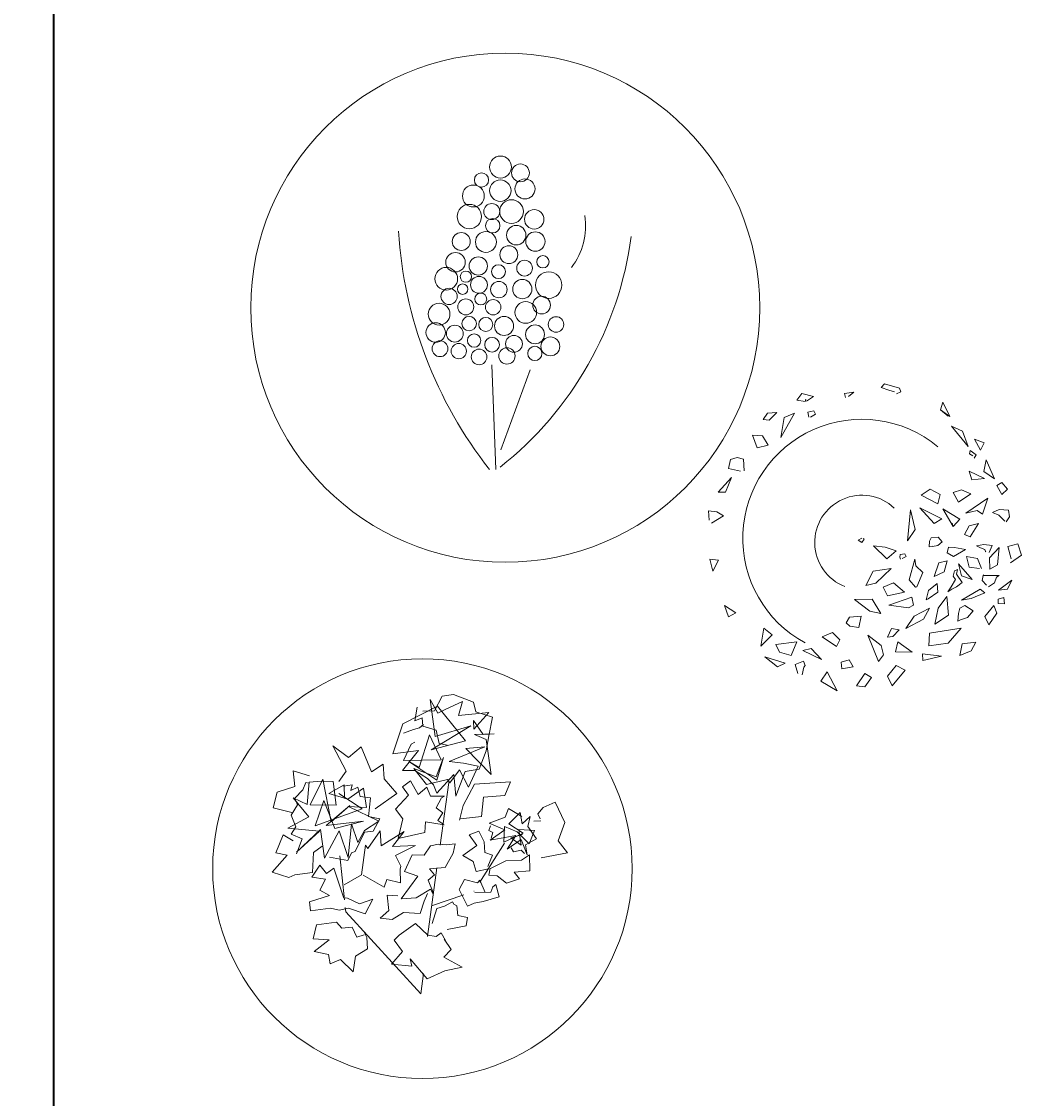
# Model space of a CAD drawing. Units: inches. Extents: x 8049 to 8459, y 820 to 1350.
# Tile 5 of 25: x 8083 to 8109, y 877 to 905. Entities that reach past the tile are written whole.
import ezdxf

# ---------------------------------------------------------------- set-up
doc = ezdxf.new("R2010")
doc.units = ezdxf.units.IN
doc.header["$MEASUREMENT"] = 0
for name, color, linetype, lineweight in [('A-ANNO-DIMS', 2, 'Continuous', 18), ('C-SITE-WALL', 7, 'Continuous', 35), ('zelen', 69, 'Continuous', 13)]:
    doc.layers.add(name, color=color, linetype=linetype, lineweight=lineweight)
doc.styles.get("Standard").update_dxf_attribs({"font": 'arial.ttf'})
doc.dimstyles.get("Standard").update_dxf_attribs({"dimtxt": 0.18, "dimasz": 0.18, "dimexe": 0.18, "dimexo": 0.0625, "dimgap": 0.09, "dimtad": 0, "dimtih": 1, "dimtoh": 1, "dimdec": 4, "dimzin": 0, "dimdsep": 46, "dimtxsty": 'Standard', "dimcen": 0.09, "dimadec": 0, "dimazin": 0, "dimtfac": 1, "dimtdec": 4, "dimtofl": 0, "dimtmove": 0, "dimatfit": 3, "dimfxl": 1, "dimtolj": 1, "dimtzin": 0, "dimarcsym": 0})

# ---------------------------------------------------------------- blocks, each defined once
blk = doc.blocks.new('z_05')
for p, q in [((47.7, 413.4), (29.2, 377.9)), ((74.4, 417.3), (47.7, 413.4)), ((122.3, 398.9), (74.4, 417.3)), ((36.3, 389.4), (-47, 347)), ((-12.6, 387.1), (-18.2, 353.9)), ((18.3, 405.2), (30.8, 316.1)), ((36.6, 372.7), (18.3, 405.2)), ((103.3, 306), (36.3, 389.4)), ((95.8, 400.3), (55.9, 381.9)), ((86.6, 366.4), (95.8, 400.3)), ((127.9, 375.3), (122.3, 398.9)), ((-18.2, 353.9), (-1, 361.5)), ((-1, 361.5), (0.6, 341.4)), ((29.2, 377.9), (0.9, 377.3)), ((55.9, 381.9), (36.6, 372.7)), ((158.8, 374.3), (86.6, 366.4)), ((122.8, 334.2), (158.8, 374.3)), ((168.1, 362.8), (127.9, 375.3)), ((159.1, 318.4), (168.1, 362.8)), ((-47, 347), (-70.6, 274.7)), ((-21.4, 333.2), (-6.8, 337.2)), ((-6.8, 337.2), (2.7, 345.1)), ((0.6, 341.4), (32.6, 331.6)), ((116, 342.1), (21, 284.9)), ((30.8, 316.1), (116, 342.1)), ((122.6, 354.6), (122.8, 334.2)), ((145.3, 321.4), (122.6, 354.6)), ((-45.7, 324.7), (-21.4, 333.2)), ((17, 320.7), (-8.1, 242.2)), ((44.8, 260.6), (17, 320.7)), ((32.6, 331.6), (40.3, 300)), ((124.7, 321.1), (172, 322.7)), ((153, 309.2), (124.7, 321.1)), ((172, 322.7), (145.3, 321.4)), ((152.5, 282), (159.1, 318.4)), ((-214.6, 294.2), (-182.9, 233.1)), ((-176.8, 265.8), (-214.6, 294.2)), ((-147, 291.7), (-176.8, 265.8)), ((-122.2, 232.2), (-147, 291.7)), ((-26.7, 298.1), (-45.4, 258.6)), ((-17.9, 303), (-26.7, 298.1)), ((21, 284.9), (103.3, 306)), ((40.3, 300), (59.6, 295.4)), ((63.8, 256.3), (149.6, 291.5)), ((149.6, 291.5), (103.8, 287.6)), ((103.8, 287.6), (164.9, 225.4)), ((164.9, 225.4), (153, 309.2)), ((-70.6, 274.7), (-9.7, 283.3)), ((-9.7, 283.3), (-47.6, 235.3)), ((-45.4, 258.6), (44.8, 260.6)), ((50.3, 265.9), (32.6, 220.2)), ((34.5, 212), (50.3, 265.9)), ((136.1, 238.6), (152.5, 282)), ((-309.5, 234.4), (-305.8, 197.1)), ((-270.2, 222.5), (-309.5, 234.4)), ((-182.9, 233.1), (-200.1, 208.7)), ((-93.7, 249.9), (-122.2, 232.2)), ((-92, 215.4), (-93.7, 249.9)), ((-47.6, 235.3), (-18.5, 235)), ((-32.2, 256.7), (34.5, 212)), ((-8.1, 242.2), (-32.2, 256.7)), ((-20.6, 240.2), (9.6, 201.8)), ((32.6, 220.2), (-20.6, 240.2)), ((-18.5, 235), (12, 215.9)), ((98.5, 252.7), (63.8, 256.3)), ((65.9, 205.1), (89, 236.9)), ((79.7, 173.9), (102.7, 232.4)), ((89, 236.9), (110.4, 195.2)), ((133.2, 245.8), (98.5, 252.7)), ((102.7, 232.4), (136.1, 238.6)), ((110.4, 195.2), (133.2, 245.8)), ((-286.6, 188.7), (-279, 206.4)), ((-279, 206.4), (-271.8, 204.4)), ((-275.9, 153.5), (-271.1, 207)), ((-271.1, 207), (-242.8, 209.3)), ((-269.3, 152.8), (-238.3, 213.9)), ((-242.8, 209.3), (-214.2, 208.4)), ((-238.3, 213.9), (-219, 112.4)), ((-214.2, 208.4), (-206.8, 152.2)), ((-61.3, 180), (-92, 215.4)), ((-28.6, 209.9), (-48, 196.2)), ((-10, 177.5), (-28.6, 209.9)), ((9.6, 201.8), (59.9, 213.6)), ((12, 215.9), (26.8, 200.5)), ((34.5, 180.8), (74.9, 225.8)), ((59.9, 213.6), (65.9, 205.1)), ((74.9, 225.8), (79.7, 173.9)), ((211.1, 208.1), (125, 202.6)), ((197.5, 175.4), (211.1, 208.1)), ((-348.1, 183.4), (-357.4, 145.5)), ((-305.8, 197.1), (-348.1, 183.4)), ((-305.7, 168.7), (-286.6, 188.7)), ((-187.8, 200.8), (-224.5, 180.1)), ((-188.9, 197.7), (-168.6, 200.5)), ((-187, 168.3), (-187.8, 200.8)), ((-178.5, 166), (-140.9, 192.9)), ((-168.6, 200.5), (-171.2, 187.4)), ((-171.2, 187.4), (-155.1, 195.5)), ((-155.1, 195.5), (-149.1, 172.6)), ((-140.9, 192.9), (-133.8, 146.3)), ((-48, 196.2), (-33.6, 175.7)), ((10.9, 194.8), (-10, 177.5)), ((19.4, 173.3), (10.9, 194.8)), ((26.8, 200.5), (34.5, 180.8)), ((42.3, 56.3), (63, 206.2)), ((125, 202.6), (98, 151)), ((-309.5, 169.9), (-275.9, 153.5)), ((-272.4, 123.9), (-309.5, 169.9)), ((-299.4, 152.8), (-305.7, 168.7)), ((-236.2, 163), (-257.1, 102.9)), ((-210, 96), (-236.2, 163)), ((-224.5, 180.1), (-178.5, 166)), ((-144.4, 143), (-200.5, 180.1)), ((-149.1, 172.6), (-124.4, 169.6)), ((-124.4, 169.6), (-129.3, 125.2)), ((-113.4, 143.1), (-61.3, 180)), ((-33.6, 175.7), (-64.3, 142.3)), ((53.3, 173.7), (19.4, 173.3)), ((33.2, 145.5), (45.7, 169.6)), ((45.7, 169.6), (53.3, 173.7)), ((141.3, 124.8), (146.2, 170.9)), ((146.2, 170.9), (197.5, 175.4)), ((318.2, 159), (289, 146.8)), ((341.6, 110.1), (318.2, 159)), ((-357.4, 145.5), (-313.2, 134.2)), ((-314.6, 127.8), (-299.4, 152.8)), ((-206.8, 152.2), (-269.3, 152.8)), ((-257.1, 102.9), (-144.4, 143)), ((-174.3, 151.5), (-230.4, 103.2)), ((-219, 112.4), (-174.3, 151.5)), ((-177.2, 148.6), (-104.7, 113.7)), ((-133.8, 146.3), (-177.2, 148.6)), ((-64.3, 142.3), (-46.8, 118.9)), ((49.2, 133.6), (33.2, 145.5)), ((36.7, 115.6), (49.2, 133.6)), ((98, 151), (88.7, 115.9)), ((198.5, 123.6), (206.2, 144.3)), ((206.2, 144.3), (238.2, 125.2)), ((207.2, 107.5), (234.5, 134.4)), ((234.5, 134.4), (238.7, 107.5)), ((289, 146.8), (276.7, 130.9)), ((276.7, 130.9), (282.3, 119)), ((-322.2, 96.6), (-272.4, 123.9)), ((-303.6, 100.1), (-314.6, 127.8)), ((-230.4, 103.2), (-141.2, 113.4)), ((-141.2, 113.4), (-210, 96)), ((-170.3, 107.2), (-177.7, 26.3)), ((-154.7, 62.5), (-170.3, 107.2)), ((-104.7, 113.7), (-138.8, 91.1)), ((-129.3, 125.2), (-102.3, 118.9)), ((-102.3, 118.9), (-117.9, 89.5)), ((-46.8, 118.9), (-58.1, 72.1)), ((5.6, 86.3), (7.6, 111.7)), ((7.6, 111.7), (51.8, 105.2)), ((48.6, 107.6), (36.7, 115.6)), ((91.6, 119.6), (141.3, 124.8)), ((159.9, 108.8), (198.5, 123.6)), ((197.7, 92.7), (159.9, 108.8)), ((241.1, 84.8), (207.2, 107.5)), ((238.7, 107.5), (258, 124.6)), ((258, 124.6), (252.2, 100.6)), ((284.1, 114.7), (267.1, 113.5)), ((324.9, 66.8), (341.6, 110.1)), ((-333.3, 80.8), (-351, 37.5)), ((-309.7, 66.5), (-333.3, 80.8)), ((-247, 90.1), (-322.2, 96.6)), ((-314.4, 82.9), (-303.6, 100.1)), ((-288, 71.4), (-314.4, 82.9)), ((-244.4, 93.4), (-301.8, 39.5)), ((-301.8, 39.5), (-247, 90.1)), ((-234.9, 25.3), (-244.4, 93.4)), ((-199.4, 90.7), (-234.9, 25.3)), ((-177.7, 26.3), (-199.4, 90.7)), ((-138.6, 87.7), (-161.1, 41.4)), ((-138.8, 91.1), (-154.7, 62.5)), ((-117.9, 89.5), (-138.6, 87.7)), ((-130.7, 48.4), (-100.9, 90.4)), ((-100.9, 90.4), (-98.5, 54.7)), ((-98.5, 54.7), (-43.7, 88.9)), ((-43.7, 88.9), (-71.8, 53.1)), ((-58.1, 72.1), (5.6, 86.3)), ((135.5, 89.5), (111.9, 81.1)), ((111.9, 81.1), (130.2, 55.1)), ((148.3, 64.3), (135.5, 89.5)), ((163.2, 102.8), (159.3, 91.6)), ((159.3, 91.6), (169, 86.6)), ((162.5, 68.1), (197.7, 92.7)), ((223.6, 79.6), (162.5, 68.1)), ((169, 86.6), (165, 72.9)), ((196.9, 101.2), (195.1, 63.5)), ((195.1, 63.5), (241.1, 84.8)), ((226.8, 87.8), (196.9, 101.2)), ((203.3, 46.4), (223.6, 79.6)), ((239.5, 81.5), (211.5, 73.6)), ((255.9, 59.2), (226.8, 87.8)), ((231.3, 94), (268.9, 91.4)), ((236.9, 55.9), (231.3, 94)), ((252.2, 100.6), (273.6, 71.3)), ((268.9, 91.4), (255.9, 59.2)), ((-302, 35.3), (-288, 71.4)), ((-260.8, 38.4), (-240.2, 53.7)), ((-145.9, -14.9), (-136.6, 56.2)), ((-136.6, 56.2), (-130.7, 48.4)), ((-71.8, 53.1), (-16.6, 55.1)), ((-16.6, 55.1), (-64.6, 31.5)), ((19, 54.4), (4.5, 32.1)), ((38.8, 58.6), (19, 54.4)), ((57.8, 57), (38.8, 58.6)), ((78.7, 59.7), (57.8, 57)), ((73.6, 37.4), (78.7, 59.7)), ((130.2, 55.1), (97.1, 31.2)), ((137.3, -32.7), (196.8, 60.8)), ((149.9, 38.3), (148.3, 64.3)), ((236.3, 69.4), (203.3, 46.4)), ((211.5, 73.6), (236.9, 55.9)), ((250.9, 32.9), (236.3, 69.4)), ((273.6, 71.3), (246.7, 57.2)), ((246.7, 57.2), (250.9, 32.9)), ((347.5, 37.8), (324.9, 66.8)), ((-324.2, 32.6), (-360.1, -8.6)), ((-351, 37.5), (-324.2, 32.6)), ((-263.3, -9.2), (-260.8, 38.4)), ((-179.1, 19.6), (-222.6, 27.6)), ((-197.6, 30.4), (-186.7, -75.1)), ((-170.2, 37.7), (-179.1, 19.6)), ((-161.1, 41.4), (-170.2, 37.7)), ((-64.6, 31.5), (-51.4, 5.7)), ((-24.4, 33.3), (-43.1, -6.5)), ((4.5, 32.1), (-24.4, 33.3)), ((54.6, 2.8), (73.6, 37.4)), ((97.1, 31.2), (121.2, 16.7)), ((168.1, 32.5), (149.9, 38.3)), ((156.5, 4.8), (168.1, 32.5)), ((218.6, 40.3), (212.6, 49.9)), ((236.5, 44), (218.6, 40.3)), ((244.2, 36.6), (236.5, 44)), ((237.6, 20.3), (256.2, 32.8)), ((256.2, 32.8), (257.4, -5.3)), ((284.6, 26.2), (347.5, 37.8)), ((-246.1, 8.6), (-264.6, -20.3)), ((-229.7, -11.4), (-246.1, 8.6)), ((-212.5, 1.1), (-229.7, -11.4)), ((-188.1, -70.9), (-212.5, 1.1)), ((-51.4, 5.7), (-53.3, -1)), ((12.2, -162.5), (34.8, 2)), ((17.3, -0.7), (54.6, 2.8)), ((121.2, 16.7), (128.5, -6.7)), ((159.5, -16), (162.4, 0.9)), ((163.5, 0), (199.5, 18.3)), ((199.5, 18.3), (237.6, 20.3)), ((-360.1, -8.6), (-319.8, -21.4)), ((-319.8, -21.4), (-305.8, -15)), ((-305.8, -15), (-263.3, -9.2)), ((-264.6, -20.3), (-232.2, -25.5)), ((-232.2, -25.5), (-245.8, -51.9)), ((-187.7, -38.6), (-145.9, -14.9)), ((-91.7, -44.5), (-142, -16)), ((-53.3, -1), (-52.3, -34)), ((-11.2, -18.3), (-50.9, -72.3)), ((-43.1, -6.5), (-11.2, -18.3)), ((14.1, -27.4), (28.8, -14.9)), ((28.8, -14.9), (17.3, -0.7)), ((128.5, -6.7), (158.7, -0.6)), ((179.2, -17.2), (159.5, -16)), ((201.2, -35.1), (179.2, -17.2)), ((232.4, -24.4), (201.2, -35.1)), ((257.4, -5.3), (219.7, -8.5)), ((219.7, -8.5), (232.4, -24.4)), ((-85.5, -25.9), (-91.7, -44.5)), ((-52.3, -34), (-85.5, -25.9)), ((-15.2, -70.2), (19.4, -49.1)), ((25.9, -56.8), (14.1, -27.4)), ((19.4, -49.1), (24.6, -59.5)), ((88.3, -50.2), (101.1, -26.2)), ((107.8, -89.9), (88.3, -50.2)), ((101.1, -26.2), (131.6, -34.3)), ((131.6, -34.3), (137.9, -27.4)), ((137.9, -27.4), (150.4, -57.2)), ((163.6, -56.6), (168.4, -43.5)), ((168.4, -43.5), (176.2, -37.8)), ((176.2, -37.8), (183.5, -67.3)), ((-222.9, -64.1), (-270.2, -79.3)), ((-245.8, -51.9), (-222.9, -64.1)), ((-179.4, -70.6), (-185, -70.2)), ((-151.1, -84.7), (-179.4, -70.6)), ((-119.1, -72.9), (-151.1, -84.7)), ((-137, -108.6), (-119.1, -72.9)), ((-84.6, -63.8), (-80.4, -99.9)), ((-59, -65.1), (-84.6, -63.8)), ((-50.9, -72.3), (-15.2, -70.2)), ((3.9, -77.8), (12.1, -59.8)), ((99.1, -62.5), (22.1, -89.1)), ((123.4, -54.1), (123.7, -54)), ((125.8, -57.1), (163.6, -56.6)), ((183.5, -67.3), (145.4, -78.6)), ((-270.2, -79.3), (-268.3, -101.3)), ((-268.3, -101.3), (-219.9, -94.9)), ((-219.9, -94.9), (-199.8, -99.2)), ((-199.8, -99.2), (-177.4, -94.6)), ((-184.9, -93), (-183.8, -103.6)), ((-177.4, -94.6), (-137, -108.6)), ((-80.4, -99.9), (-101.4, -118.3)), ((-5.1, -107.6), (3.9, -77.8)), ((34.7, -95.4), (23.5, -131.1)), ((52.8, -90), (34.7, -95.4)), ((72.1, -79.9), (52.8, -90)), ((75, -85.4), (72.1, -79.9)), ((82.5, -89.1), (75, -85.4)), ((85.1, -112.3), (82.5, -89.1)), ((124.2, -82.4), (107.8, -89.9)), ((145.4, -78.6), (124.2, -82.4)), ((-205.8, -128), (-253.7, -134.6)), ((-192.7, -142.7), (-205.8, -128)), ((-183.8, -103.6), (-3.6, -299.6)), ((-101.4, -118.3), (-72.6, -121.5)), ((-72.6, -121.5), (-45.6, -105.4)), ((-45.6, -105.4), (-5.1, -107.6)), ((108, -117.3), (85.1, -112.3)), ((104.9, -137.2), (108, -117.3)), ((-253.7, -134.6), (-261.4, -168.3)), ((-168.7, -140.1), (-192.7, -142.7)), ((-157, -164.4), (-168.7, -140.1)), ((-133.5, -165.3), (-138.4, -154.1)), ((-16.2, -131.7), (-55.5, -159.5)), ((13.1, -159.3), (-16.2, -131.7)), ((45, -154.1), (32.6, -162.8)), ((55.2, -172.3), (45, -154.1)), ((59.4, -145.7), (104.9, -137.2)), ((-261.4, -168.3), (-223.5, -170.8)), ((-223.5, -170.8), (-259.2, -198.1)), ((-139.9, -158.9), (-157, -164.4)), ((-131.8, -192.3), (-133.5, -165.3)), ((-55.5, -159.5), (-67.8, -171.1)), ((-67.8, -171.1), (-47.6, -198.1)), ((32.6, -162.8), (13.1, -159.3)), ((69.1, -193.4), (52.3, -169.2)), ((-259.2, -198.1), (-224.7, -206)), ((-224.7, -206), (-221.4, -228.1)), ((-160.4, -209.4), (-131.8, -192.3)), ((-47.6, -198.1), (-74.3, -229.2)), ((51.3, -211.7), (69.1, -193.4)), ((-221.4, -228.1), (-196.4, -217.5)), ((-196.4, -217.5), (-166.3, -247.2)), ((-166.3, -247.2), (-160.4, -209.4)), ((-74.3, -229.2), (-25.6, -233.9)), ((-29.7, -216.4), (11.5, -264)), ((-25.6, -233.9), (-29.7, -216.4)), ((95.2, -236.2), (51.3, -211.7)), ((2.5, -250.9), (-3.6, -299.6)), ((11.5, -264), (54, -244.9)), ((54, -244.9), (95.2, -236.2))]:
    blk.add_line(p, q)
blk.add_circle((0, 0), 502.5)
blk = doc.blocks.new('z_06')
for p, q in [((-26, -111.8), (-18.2, -317.4)), ((48.7, -121.5), (-8.6, -278.6))]:
    blk.add_line(p, q)
for centre, radius in [((0, 0), 499.1), ((-9.3, 275.8), 21.5), ((29.8, 264.3), 17.5), ((-46.5, 250.4), 14), ((-62.5, 219), 21.4), ((-9.7, 229.6), 21.1), ((38.7, 232.9), 19.7), ((12.3, 188.5), 23.2), ((-70.3, 178.8), 23.9), ((-26.4, 188.5), 15.7), ((56.9, 173.3), 19), ((-24.6, 160.8), 14.2), ((-37.9, 128.9), 20.5), ((21.6, 142.3), 19.1), ((59.1, 129.8), 19), ((-86.3, 129.8), 17.6), ((-97.5, 89.2), 19.1), ((7.1, 104), 17.6), ((-52.8, 81.8), 18), ((37.9, 77.6), 15.4), ((74, 90.1), 12), ((-115.7, 56.8), 22.2), ((-77, 60.9), 11.1), ((-13.1, 70.7), 13.7), ((85.2, 44.4), 26), ((-83.5, 36.4), 10.2), ((-51.5, 44.9), 16.6), ((-12.5, 35.6), 16.1), ((33.5, 36.5), 18.9), ((-110.1, 22.2), 15.9), ((-47.9, 17.1), 11.7), ((71.4, 5.1), 17.3), ((-129.8, -12.5), 21.4), ((-77.3, 1.7), 15.7), ((-23.7, 1), 15.1), ((40.2, -9.2), 21.3), ((-70.8, -31.2), 14.2), ((-38.2, -32.7), 13.7), ((-2.3, -35.8), 18.7), ((99.7, -32.8), 15.2), ((-136.5, -48.5), 19.1), ((-98.8, -50.8), 16.5), ((58.4, -52.2), 18.5), ((-61.1, -64.4), 13.1), ((-25.8, -72.6), 14.4), ((17.1, -70.7), 16.5), ((88.5, -75.8), 18.5), ((-128, -80.4), 15.5), ((-91.1, -85.1), 15), ((-51.3, -96.5), 15.3), ((3.4, -94.5), 16), ((58, -89.6), 14)]:
    blk.add_circle(centre, radius)
for centre, radius, start, end in [((21.1, 161.1), 136.5, 323.03, 8.2301), ((631.6, 203.5), 842.7, 183.6263, 218.177), ((-440.2, 231.1), 693.3, 308.3911, 352.4108)]:
    blk.add_arc(centre, radius, start, end)
blk = doc.blocks.new('z_66')
for p, q in [((83.2, 488.9), (72.7, 477.7)), ((72.7, 477.7), (96.4, 469.7)), ((129.8, 476.2), (83.2, 488.9)), ((134, 464.6), (129.8, 476.2)), ((-176.4, 458.5), (-191.7, 438.6)), ((-191.7, 438.6), (-165.6, 433.5)), ((-139.2, 449.4), (-176.4, 458.5)), ((-165.6, 433.5), (-163.6, 441.1)), ((-161.1, 434.6), (-139.2, 449.4)), ((-13.6, 463.6), (-42.5, 459.2)), ((-42.5, 459.2), (-39.3, 446.9)), ((-30.3, 449.4), (-13.6, 463.6)), ((96.4, 469.7), (114.5, 463.9)), ((114.5, 463.9), (114.5, 463.9)), ((120.4, 457.8), (134, 464.6)), ((-165.6, 433.5), (-165.6, 433.5)), ((-138.9, 404.9), (-156.9, 400.2)), ((-133.3, 394.8), (-138.9, 404.9)), ((265.2, 432.1), (258.2, 407.5)), ((258.2, 407.5), (287.4, 387.2)), ((258.2, 407.5), (281.9, 388.6)), ((287.4, 387.2), (265.2, 432.1)), ((-283.6, 397.7), (-297.2, 378.2)), ((-297.2, 378.2), (-277.7, 376)), ((-254, 399.9), (-283.6, 397.7)), ((-277.7, 376), (-272.8, 380.7)), ((-272.8, 380.7), (-254, 399.9)), ((-241.9, 321.7), (-199.1, 397.3)), ((-231.4, 383.6), (-241.9, 321.7)), ((-199.1, 397.3), (-231.4, 383.6)), ((-156.9, 400.2), (-153.8, 385.4)), ((-148.6, 384.7), (-133.3, 394.8)), ((281.9, 388.6), (281.9, 388.6)), ((344.2, 293.1), (292, 357.2)), ((292, 357.2), (326.8, 341.2)), ((326.8, 341.2), (344.2, 293.1)), ((-330.3, 328.9), (-298.6, 327.1)), ((-316, 288.8), (-330.3, 328.9)), ((-298.6, 327.1), (-280.8, 297.1)), ((383.1, 281.9), (364.4, 316.3)), ((364.4, 316.3), (394.6, 305.1)), ((394.6, 305.1), (383.1, 281.9)), ((-280.8, 297.1), (-316, 288.8)), ((350.8, 280.8), (348.7, 270.3)), ((348.7, 270.3), (358.8, 264.5)), ((369.2, 266.7), (350.8, 280.8)), ((-399.2, 252.6), (-405.8, 224)), ((-377.9, 259.1), (-399.2, 252.6)), ((-358.4, 254), (-377.9, 259.1)), ((-356, 217.5), (-358.4, 254)), ((358.8, 264.5), (358.8, 264.5)), ((363.3, 256.6), (369.2, 266.7)), ((400.9, 251.9), (393.9, 214.6)), ((426.6, 192.2), (400.9, 251.9)), ((-405.8, 224), (-368.2, 216.4)), ((-368.2, 216.4), (-368.2, 216.4)), ((348, 215.7), (356, 188.9)), ((395.3, 193.2), (348, 215.7)), ((393.9, 214.6), (426.6, 192.2)), ((-396.4, 196.1), (-438.1, 150.2)), ((-414.8, 150.9), (-396.4, 196.1)), ((356, 188.9), (395.3, 193.2)), ((450, 180.6), (434.3, 171.2)), ((434.3, 171.2), (449.6, 142.6)), ((467.7, 160.3), (450, 180.6)), ((-438.1, 150.2), (-414.8, 150.9)), ((225.2, 159.9), (197, 140.8)), ((197, 140.8), (249.5, 113.6)), ((256.8, 142.6), (225.2, 159.9)), ((249.5, 113.6), (256.8, 142.6)), ((323.6, 157.8), (297.5, 149.8)), ((297.5, 149.8), (314.6, 119.4)), ((314.6, 119.4), (352.9, 145.5)), ((352.9, 145.5), (323.6, 157.8)), ((449.6, 142.6), (467.7, 160.3)), ((193.1, 101.3), (238, 52.1)), ((261.7, 66.6), (193.1, 101.3)), ((336.9, 84.3), (405.8, 131.7)), ((405.8, 131.7), (389.8, 82.1)), ((-468.4, 91.6), (-466.3, 62.6)), ((-441.6, 89), (-468.4, 91.6)), ((-458.3, 53.9), (-421.1, 76)), ((-421.1, 76), (-441.6, 89)), ((164.3, 94.8), (154.2, -2.2)), ((178.9, 33.3), (164.3, 94.8)), ((265.2, 98.8), (297.2, 42.7)), ((318.8, 66.2), (265.2, 98.8)), ((372.7, 93), (336.9, 84.3)), ((389.8, 82.1), (372.7, 93)), ((441.6, 95.9), (420.7, 86.5)), ((420.7, 86.5), (440.2, 78.5)), ((440.2, 78.5), (459.7, 59.7)), ((470.5, 93.7), (441.6, 95.9)), ((463.2, 57.9), (474, 73.5)), ((474, 73.5), (470.5, 93.7)), ((-466.3, 62.6), (-466.3, 62.6)), ((238, 52.1), (261.7, 66.6)), ((297.2, 42.7), (294.1, 53.6)), ((297.2, 42.7), (318.8, 66.2)), ((347.3, 45.2), (332.7, 18.1)), ((376.9, 52.5), (347.3, 45.2)), ((350.8, 10.9), (376.9, 52.5)), ((459.7, 59.7), (459.7, 59.7)), ((11.8, 6.2), (0, 0)), ((0, 0), (12.2, -6.9)), ((12.2, -6.9), (19.1, 2.9)), ((19.1, 2.9), (15.7, 5.8)), ((154.2, -2.2), (178.9, 33.3)), ((229, 7.2), (223.1, -2.5)), ((250.6, 9.8), (229, 7.2)), ((263.4, -5.4), (250.6, 9.8)), ((332.7, 18.1), (350.8, 10.9)), ((84.6, -21.7), (48, -17)), ((48, -17), (90.1, -58.3)), ((119.4, -32.9), (84.6, -21.7)), ((90.1, -58.3), (119.4, -32.9)), ((223.1, -2.5), (222.7, -20.6)), ((222.7, -20.6), (234.2, -18.1)), ((233.2, -19.9), (249.9, -15.9)), ((234.2, -18.1), (234.2, -18.1)), ((249.9, -15.9), (263.4, -5.4)), ((282.9, -21.3), (279.1, -39.1)), ((302.1, -22.8), (282.9, -21.3)), ((298.6, -50.3), (335.8, -28.6)), ((335.8, -28.6), (302.1, -22.8)), ((393.6, -13), (371, -17)), ((371, -17), (383.5, -23.5)), ((383.5, -23.5), (396.7, -28.9)), ((420, -15.9), (393.6, -13)), ((396.7, -28.9), (398.5, -35.5)), ((410.3, -38), (420, -15.9)), ((442, -22.4), (411.3, -55.4)), ((436, -77.1), (442, -22.4)), ((499.7, -10.9), (468.8, -19.9)), ((468.8, -19.9), (478.8, -58.6)), ((510.9, -47), (499.7, -10.9)), ((-464.2, -59.3), (-436.4, -62.6)), ((-454.5, -96.3), (-464.2, -59.3)), ((-436.4, -62.6), (-454.5, -96.3)), ((131.9, -44.9), (130.2, -52.5)), ((130.2, -52.5), (132.9, -59.3)), ((146.5, -42.3), (131.9, -44.9)), ((138.2, -56.8), (151, -51)), ((151, -51), (146.5, -42.3)), ((177.8, -59), (160.1, -123.8)), ((181, -80.3), (177.8, -59)), ((278.4, -64), (252.6, -70.9)), ((269.7, -98.4), (278.4, -64)), ((279.1, -39.1), (298.6, -50.3)), ((339, -51), (347.7, -84.3)), ((374.1, -56.8), (339, -51)), ((386.3, -87.9), (374.1, -56.8)), ((398.5, -35.5), (399.5, -35.8)), ((411.3, -55.4), (412.7, -90.8)), ((477.5, -70.2), (510.9, -47)), ((478.8, -58.6), (478.8, -58.6)), ((47.7, -96.6), (24, -141.9)), ((104.1, -87.9), (47.7, -96.6)), ((56, -133.9), (104.1, -87.9)), ((202.2, -100.6), (181, -80.3)), ((183.7, -145.5), (202.2, -100.6)), ((252.6, -70.9), (237.7, -112.9)), ((237.7, -112.9), (269.7, -98.4)), ((301.7, -95.5), (297.9, -112.2)), ((310.8, -91.9), (301.7, -95.5)), ((307.6, -106), (310.8, -91.9)), ((314.2, -74.2), (356.7, -123)), ((323.3, -111.1), (314.2, -74.2)), ((347.7, -84.3), (379.7, -88.3)), ((379.7, -88.3), (379.7, -88.3)), ((412.7, -90.8), (436, -77.1)), ((24, -141.9), (56, -133.9)), ((111.4, -132.8), (78.3, -146.2)), ((145.1, -162.1), (111.4, -132.8)), ((160.1, -123.8), (179.6, -146.6)), ((304.5, -123), (291.6, -145.8)), ((297.9, -112.2), (304.5, -123)), ((325.4, -132.4), (307.6, -106)), ((308.3, -145.8), (325.4, -132.4)), ((356.7, -123), (323.3, -111.1)), ((356.7, -123), (356.7, -123)), ((356.7, -123), (356.7, -123)), ((391.2, -110), (388.4, -125.6)), ((388.4, -125.6), (402.3, -140.8)), ((391.2, -110), (393.2, -108.6)), ((441.3, -110), (391.2, -110)), ((407.9, -145.5), (427, -133.5)), ((427, -133.5), (432.9, -115.8)), ((432.9, -115.8), (441.3, -110)), ((480.9, -124.5), (439.2, -156)), ((467.7, -153.4), (480.9, -124.5)), ((78.3, -146.2), (92.2, -174.1)), ((92.2, -174.1), (145.1, -162.1)), ((179.6, -146.6), (183.7, -145.5)), ((220.6, -157), (212.6, -186)), ((219.2, -183.5), (249.2, -162.1)), ((247.1, -135.7), (220.6, -157)), ((249.2, -162.1), (247.1, -135.7)), ((291.6, -145.8), (281.2, -161.8)), ((281.2, -161.8), (293, -152.7)), ((293, -152.7), (308.3, -145.8)), ((382.5, -152.7), (323.3, -187.4)), ((353.9, -182), (396.7, -164.3)), ((396.7, -164.3), (382.5, -152.7)), ((402.3, -140.8), (402.3, -140.8)), ((439.2, -156), (467.7, -153.4)), ((44.5, -184.2), (-10.8, -184.9)), ((-10.8, -184.9), (36.9, -222.2)), ((71, -229.1), (44.5, -184.2)), ((168.1, -178.4), (96.7, -202.6)), ((173, -203.4), (168.1, -178.4)), ((212.6, -186), (219.2, -183.5)), ((277.4, -176.2), (250.2, -212.4)), ((283.3, -233.8), (277.4, -176.2)), ((323.3, -187.4), (353.9, -182)), ((438.5, -183.8), (456.2, -179.1)), ((438.5, -197.6), (438.5, -183.8)), ((458.7, -199), (438.5, -197.6)), ((456.2, -179.1), (458.7, -199)), ((-417.9, -204.1), (-405.1, -239.6)), ((-382.8, -226.5), (-417.9, -204.1)), ((-405.1, -239.6), (-382.8, -226.5)), ((36.9, -222.2), (71, -229.1)), ((96.7, -202.6), (157.6, -211.3)), ((157.6, -211.3), (173, -203.4)), ((223.8, -212.4), (175.4, -237.7)), ((204.3, -246.8), (223.8, -212.4)), ((250.2, -212.4), (240.1, -262.4)), ((240.1, -262.4), (283.3, -233.8)), ((314.6, -228.7), (311.8, -252.6)), ((318.4, -212.1), (314.6, -228.7)), ((334.1, -203.7), (318.4, -212.1)), ((360.2, -221.1), (334.1, -203.7)), ((342.8, -241.4), (360.2, -221.1)), ((425.3, -204.5), (396.7, -238.5)), ((409.2, -264.2), (434.3, -228)), ((434.3, -228), (425.3, -204.5)), ((-26.4, -240.3), (-37.6, -258.4)), ((-37.6, -258.4), (-25.8, -268.5)), ((10.1, -237.7), (-26.4, -240.3)), ((-25.8, -268.5), (2.4, -273.2)), ((-25.8, -268.5), (-25.8, -268.5)), ((-25.8, -268.5), (-25.8, -268.5)), ((2.4, -273.2), (10.1, -237.7)), ((175.4, -237.7), (149.6, -276.1)), ((149.6, -276.1), (204.3, -246.8)), ((311.8, -252.6), (320.5, -249.3)), ((320.5, -249.3), (342.8, -241.4)), ((396.7, -238.5), (409.2, -264.2)), ((-295.1, -275), (-304.2, -331.5)), ((-304.2, -331.5), (-269, -296)), ((-269, -296), (-295.1, -275)), ((-80, -288), (-112.4, -302.5)), ((-112.4, -302.5), (-67.5, -331.8)), ((-56.7, -311.6), (-80, -288)), ((30.6, -297.1), (72.7, -329.3)), ((64, -379.6), (30.6, -297.1)), ((105.1, -276.1), (91.9, -303.6)), ((91.9, -303.6), (108.6, -301.4)), ((128.8, -280.4), (105.1, -276.1)), ((108.6, -301.4), (128.8, -280.4)), ((223.8, -290.2), (221.3, -330)), ((322.2, -275), (223.8, -290.2)), ((282.2, -321.7), (322.2, -275)), ((-191.1, -317.4), (-256.8, -326.4)), ((-256.8, -326.4), (-245.7, -350.3)), ((-209.8, -360.4), (-191.1, -317.4)), ((-67.5, -331.8), (-56.7, -311.6)), ((72.7, -329.3), (79.3, -357.9)), ((117.3, -348.8), (124.2, -317.7)), ((124.2, -317.7), (168.8, -349.9)), ((221.3, -330), (282.2, -321.7)), ((325.7, -323.9), (318.4, -360.1)), ((368.9, -319.2), (325.7, -323.9)), ((354.3, -346.3), (368.9, -319.2)), ((-292, -364.4), (-252, -395.5)), ((-228.3, -383.9), (-292, -364.4)), ((-245.7, -350.3), (-209.8, -360.4)), ((-172.6, -344.9), (-146.9, -338.7)), ((-114.8, -372.7), (-172.6, -344.9)), ((-146.9, -338.7), (-114.8, -372.7)), ((79.3, -357.9), (64, -379.6)), ((168.8, -349.9), (117.3, -348.8)), ((201.8, -355), (202.2, -376.3)), ((261, -362.2), (201.8, -355)), ((202.2, -376.3), (261, -362.2)), ((318.4, -360.1), (354.3, -346.3)), ((-252, -395.5), (-228.3, -383.9)), ((-197.3, -388.3), (-171.2, -377.8)), ((-188.3, -416.9), (-197.3, -388.3)), ((-169.5, -396.6), (-174.7, -420.5)), ((-171.2, -377.8), (-166, -391.5)), ((-166, -391.5), (-169.5, -396.6)), ((-27.8, -374.5), (-52.9, -381.8)), ((-52.9, -381.8), (-50.8, -402)), ((-50.8, -402), (-15.3, -396.2)), ((-15.3, -396.2), (-27.8, -374.5)), ((91.9, -424.8), (119, -391.5)), ((119, -391.5), (146.9, -406.4)), ((-174.7, -420.5), (-174.7, -420.5)), ((-116.2, -441.1), (-96.4, -411.8)), ((-96.4, -411.8), (-65.8, -470.8)), ((21.6, -417.2), (-4.5, -455.6)), ((42.1, -428.8), (21.6, -417.2)), ((21.6, -458.1), (42.1, -428.8)), ((106.8, -455.6), (91.9, -424.8)), ((146.9, -406.4), (106.8, -455.6)), ((-65.8, -470.8), (-116.2, -441.1)), ((-4.5, -455.6), (21.6, -458.1))]:
    blk.add_line(p, q)
for centre, radius, start, end in [((11.8, 6.2), 372.3, 50.2118, 241.5185), ((12.2, -6.9), 147.8, 46.7611, 248.9067)]:
    blk.add_arc(centre, radius, start, end)
blk = doc.blocks.new('*D50')
at = {"layer": 'A-ANNO-DIMS', "color": 0, "lineweight": -2, "transparency": 16777216}
for p, q in [((8083.335, 1045.871), (8049.617, 1045.871)), ((8049.797, 1045.691), (8049.797, 945.553)), ((8049.797, 845.051), (8049.797, 945.189)), ((8074.335, 844.871), (8049.617, 844.871))]:
    blk.add_line(p, q, dxfattribs=at)
at = {"layer": 'A-ANNO-DIMS', "color": 0, "transparency": 16777216}
for points in [[(8049.767, 1045.691), (8049.827, 1045.691), (8049.797, 1045.871)], [(8049.767, 845.051), (8049.827, 845.051), (8049.797, 844.871)]]:
    blk.add_solid(points, dxfattribs=at)
at = {"layer": 'Defpoints', "color": 0, "transparency": 16777216}
for p in [(8049.797, 1045.871), (8083.397, 1045.871), (8074.397, 844.871)]:
    blk.add_point(p, dxfattribs=at)
at = {"layer": 'A-ANNO-DIMS', "color": 0, "transparency": 16777216, "insert": (8049.797, 945.371), "char_height": 0.18, "attachment_point": 5}
blk.add_mtext('\\A1;201', dxfattribs=at)
blk = doc.blocks.new('*D70')
at = {"layer": 'A-ANNO-DIMS', "color": 0, "lineweight": -2, "transparency": 16777216}
for p, q in [((8083.397, 1045.808), (8083.397, 820.091)), ((8137.397, 1045.808), (8137.397, 820.091)), ((8083.577, 820.271), (8110.179, 820.271)), ((8137.217, 820.271), (8110.616, 820.271))]:
    blk.add_line(p, q, dxfattribs=at)
at = {"layer": 'A-ANNO-DIMS', "color": 0, "transparency": 16777216}
for points in [[(8083.577, 820.301), (8083.577, 820.241), (8083.397, 820.271)], [(8137.217, 820.301), (8137.217, 820.241), (8137.397, 820.271)]]:
    blk.add_solid(points, dxfattribs=at)
at = {"layer": 'Defpoints', "color": 0, "transparency": 16777216}
for p in [(8083.397, 1045.871), (8137.397, 1045.871), (8083.397, 820.271)]:
    blk.add_point(p, dxfattribs=at)
at = {"layer": 'A-ANNO-DIMS', "color": 0, "transparency": 16777216, "insert": (8110.397, 820.271), "char_height": 0.18, "attachment_point": 5}
blk.add_mtext('\\A1;54', dxfattribs=at)
blk = doc.blocks.new('*D76')
at = {"layer": 'A-ANNO-DIMS', "color": 0, "lineweight": -2, "transparency": 16777216}
for p, q in [((8083.397, 1054.808), (8083.397, 820.091)), ((8299.397, 1054.808), (8299.397, 820.091)), ((8083.577, 820.271), (8191.107, 820.271)), ((8299.217, 820.271), (8191.688, 820.271))]:
    blk.add_line(p, q, dxfattribs=at)
at = {"layer": 'A-ANNO-DIMS', "color": 0, "transparency": 16777216}
for points in [[(8083.577, 820.301), (8083.577, 820.241), (8083.397, 820.271)], [(8299.217, 820.301), (8299.217, 820.241), (8299.397, 820.271)]]:
    blk.add_solid(points, dxfattribs=at)
at = {"layer": 'Defpoints', "color": 0, "transparency": 16777216}
for p in [(8083.397, 1054.871), (8299.397, 1054.871), (8299.397, 820.271)]:
    blk.add_point(p, dxfattribs=at)
at = {"layer": 'A-ANNO-DIMS', "color": 0, "transparency": 16777216, "insert": (8191.397, 820.271), "char_height": 0.18, "attachment_point": 5}
blk.add_mtext('\\A1;216', dxfattribs=at)
blk = doc.blocks.new('*D88')
at = {"layer": 'A-ANNO-DIMS', "color": 0, "lineweight": -2, "transparency": 16777216}
for p, q in [((8083.397, 1162.808), (8083.397, 820.091)), ((8139.397, 1162.808), (8139.397, 820.091)), ((8083.577, 820.271), (8111.179, 820.271)), ((8139.217, 820.271), (8111.616, 820.271))]:
    blk.add_line(p, q, dxfattribs=at)
at = {"layer": 'A-ANNO-DIMS', "color": 0, "transparency": 16777216}
for points in [[(8083.577, 820.301), (8083.577, 820.241), (8083.397, 820.271)], [(8139.217, 820.301), (8139.217, 820.241), (8139.397, 820.271)]]:
    blk.add_solid(points, dxfattribs=at)
at = {"layer": 'Defpoints', "color": 0, "transparency": 16777216}
for p in [(8083.397, 1162.871), (8139.397, 1162.871), (8139.397, 820.271)]:
    blk.add_point(p, dxfattribs=at)
at = {"layer": 'A-ANNO-DIMS', "color": 0, "transparency": 16777216, "insert": (8111.397, 820.271), "char_height": 0.18, "attachment_point": 5}
blk.add_mtext('\\A1;56', dxfattribs=at)

msp = doc.modelspace()

# ---------------------------------------------------------------- linework, layer by layer
at = {"layer": 'C-SITE-WALL'}
msp.add_line((8083.3974, 1315.8706), (8083.3974, 853.8706), dxfattribs=at)

# ---------------------------------------------------------------- block references
at = {"layer": 'zelen'}
for name, p, xscale, yscale, zscale in [('z_06', (8095.0845, 897.3305), 0.0131883500742978, 0.0131883500742978, 0.0131883500742978), ('z_66', (8104.2111, 891.3183), 0.0082668533249786, 0.0082668533249786, 0.0082668533249786), ('z_05', (8092.9423, 882.828), 0.0107957317921007, 0.0107957317921007, 0.0107957317921007)]:
    msp.add_blockref(name, p, dxfattribs=dict(at, xscale=xscale, yscale=yscale, zscale=zscale))

# ---------------------------------------------------------------- dimensions: what is measured, and where the dimension line sits
at = {"layer": 'A-ANNO-DIMS'}
for base, p1, p2, picture, middle in [((8139.3974, 820.2706), (8083.3974, 1162.8706), (8139.3974, 1162.8706), '*D88', (8111.3974, 820.2706)), ((8299.3974, 820.2706), (8083.3974, 1054.8706), (8299.3974, 1054.8706), '*D76', (8191.3974, 820.2706)), ((8083.3974, 820.2706), (8137.3974, 1045.8706), (8083.3974, 1045.8706), '*D70', (8110.3974, 820.2706))]:
    dim = msp.add_linear_dim(base=base, p1=p1, p2=p2, dimstyle='Standard', override={"dimdec": 0, "dimlfac": 1, "dimrnd": 0, "dimzin": 0, "dimdsep": 46, "dimlunit": 2}, dxfattribs=at)
    dim.commit()
    dim.dimension.update_dxf_attribs({"geometry": picture, "text_midpoint": middle})
dim = msp.add_linear_dim(base=(8049.7974, 1045.8706), p1=(8074.3974, 844.8706), p2=(8083.3974, 1045.8706), angle=90, dimstyle='Standard', override={"dimdec": 0, "dimlfac": 1, "dimrnd": 0, "dimzin": 0, "dimdsep": 46, "dimlunit": 2}, dxfattribs=at)
dim.commit()
dim.dimension.update_dxf_attribs({"geometry": '*D50', "text_midpoint": (8049.7974, 945.3706)})

doc.saveas('drawing.dxf')
